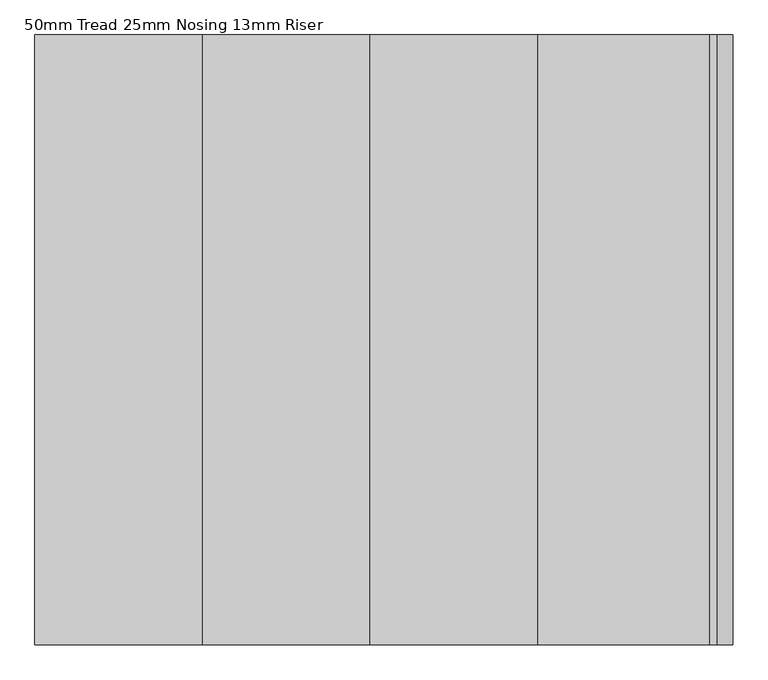
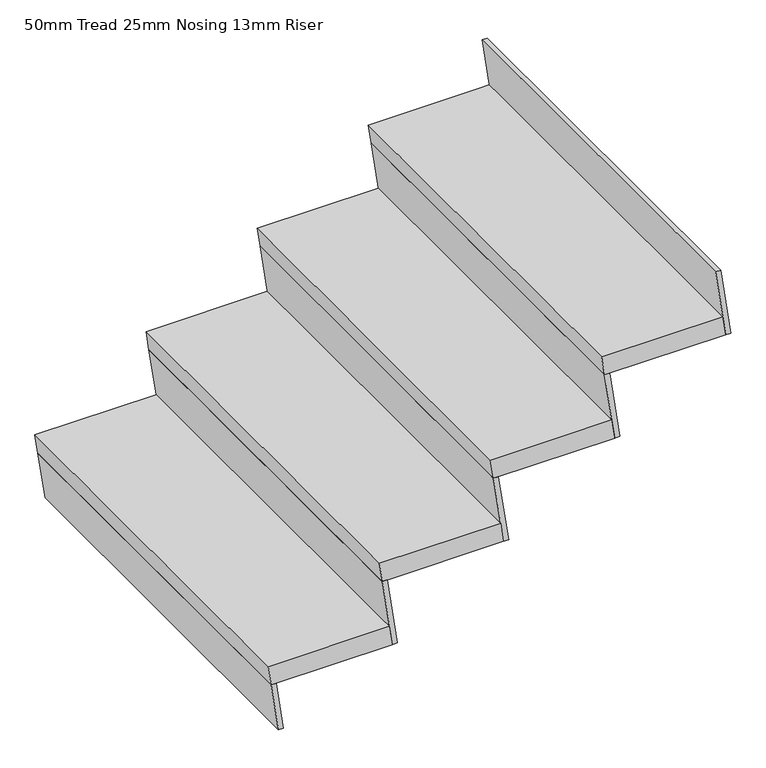
"""IFC4 building model written with IfcOpenShell, lengths in millimetres: stair flight geometry, 50mm Tread 25mm Nosing 13mm Riser."""

from ifc_helpers import new_model, si_unit, origin, place, context, project, spatial, faceted_brep, source, transform, mapped, element, save


def stair_flight_50mm_tread_25mm_nosing_13mm_riser_3ceddbfd(model_context):
    return source(origin(), model_context, "Body", "Brep", [
        faceted_brep([(-3491.9701746, -2541.1890637, 173.9130435), (-3484.7826746, -2541.1890637, 123.9130435), (-3484.7826746, -1541.1632824, 123.9130435), (-3491.9701746, -1541.1632824, 173.9130435), (-3791.9701746, -1541.1632824, 173.9130435), (-3791.9701746, -2541.1890637, 173.9130435), (-3784.7826746, -2541.1890637, 123.9130435), (-3784.7826746, -1541.1632824, 123.9130435)], [[[0, 1, 2, 3]], [[3, 4, 5, 0]], [[2, 1, 6, 7]], [[4, 3, 2, 7]], [[0, 5, 6, 1]], [[5, 4, 7, 6]]]),
        faceted_brep([(-3784.7826746, -2541.1890637, 123.9130435), (-3766.9701746, -2541.1890637, 0.0), (-3754.3416846, -2541.1890637, 0.0), (-3772.1541846, -2541.1890637, 123.9130435), (-3784.7826746, -1541.1632824, 123.9130435), (-3772.1541846, -1541.1632824, 123.9130435), (-3754.3416846, -1541.1632824, 0.0), (-3766.9701746, -1541.1632824, 0.0)], [[[0, 1, 2, 3]], [[4, 5, 6, 7]], [[1, 0, 4, 7]], [[2, 1, 7, 6]], [[3, 2, 6, 5]], [[0, 3, 5, 4]]]),
        faceted_brep([(-3509.7826746, -2541.1890637, 297.826087), (-3484.7826746, -2541.1890637, 123.9130435), (-3472.1541846, -2541.1890637, 123.9130435), (-3497.1541846, -2541.1890637, 297.826087), (-3509.7826746, -1541.1632824, 297.826087), (-3497.1541846, -1541.1632824, 297.826087), (-3472.1541846, -1541.1632824, 123.9130435), (-3484.7826746, -1541.1632824, 123.9130435)], [[[0, 1, 2, 3]], [[4, 5, 6, 7]], [[1, 0, 4, 7]], [[2, 1, 7, 6]], [[3, 2, 6, 5]], [[0, 3, 5, 4]]]),
        faceted_brep([(-3216.9701746, -1541.1632824, 347.826087), (-3516.9701746, -1541.1632824, 347.826087), (-3516.9701746, -2541.1890637, 347.826087), (-3216.9701746, -2541.1890637, 347.826087), (-3209.7826746, -1541.1632824, 297.826087), (-3209.7826746, -2541.1890637, 297.826087), (-3509.7826746, -2541.1890637, 297.826087), (-3509.7826746, -1541.1632824, 297.826087)], [[[0, 1, 2, 3]], [[4, 5, 6, 7]], [[1, 0, 4, 7]], [[3, 2, 6, 5]], [[3, 5, 4, 0]], [[2, 1, 7, 6]]]),
        faceted_brep([(-3234.7826746, -2541.1890637, 471.7391304), (-3209.7826746, -2541.1890637, 297.826087), (-3197.1541846, -2541.1890637, 297.826087), (-3222.1541846, -2541.1890637, 471.7391304), (-3234.7826746, -1541.1632824, 471.7391304), (-3222.1541846, -1541.1632824, 471.7391304), (-3197.1541846, -1541.1632824, 297.826087), (-3209.7826746, -1541.1632824, 297.826087)], [[[0, 1, 2, 3]], [[4, 5, 6, 7]], [[1, 0, 4, 7]], [[2, 1, 7, 6]], [[3, 2, 6, 5]], [[0, 3, 5, 4]]]),
        faceted_brep([(-2941.9701746, -1541.1632824, 521.7391304), (-3241.9701746, -1541.1632824, 521.7391304), (-3241.9701746, -2541.1890637, 521.7391304), (-2941.9701746, -2541.1890637, 521.7391304), (-2934.7826746, -1541.1632824, 471.7391304), (-2934.7826746, -2541.1890637, 471.7391304), (-3234.7826746, -2541.1890637, 471.7391304), (-3234.7826746, -1541.1632824, 471.7391304)], [[[0, 1, 2, 3]], [[4, 5, 6, 7]], [[1, 0, 4, 7]], [[3, 2, 6, 5]], [[3, 5, 4, 0]], [[2, 1, 7, 6]]]),
        faceted_brep([(-2684.7826746, -2541.1890637, 819.5652174), (-2659.7826746, -2541.1890637, 645.6521739), (-2647.1541846, -2541.1890637, 645.6521739), (-2672.1541846, -2541.1890637, 819.5652174), (-2684.7826746, -1541.1632824, 819.5652174), (-2672.1541846, -1541.1632824, 819.5652174), (-2647.1541846, -1541.1632824, 645.6521739), (-2659.7826746, -1541.1632824, 645.6521739)], [[[0, 1, 2, 3]], [[4, 5, 6, 7]], [[1, 0, 4, 7]], [[2, 1, 7, 6]], [[3, 2, 6, 5]], [[0, 3, 5, 4]]]),
        faceted_brep([(-2959.7826746, -2541.1890637, 645.6521739), (-2934.7826746, -2541.1890637, 471.7391304), (-2922.1541846, -2541.1890637, 471.7391304), (-2947.1541846, -2541.1890637, 645.6521739), (-2959.7826746, -1541.1632824, 645.6521739), (-2947.1541846, -1541.1632824, 645.6521739), (-2922.1541846, -1541.1632824, 471.7391304), (-2934.7826746, -1541.1632824, 471.7391304)], [[[0, 1, 2, 3]], [[4, 5, 6, 7]], [[1, 0, 4, 7]], [[2, 1, 7, 6]], [[3, 2, 6, 5]], [[0, 3, 5, 4]]]),
        faceted_brep([(-2666.9701746, -1541.1632824, 695.6521739), (-2691.9701746, -1541.1632824, 695.6521739), (-2966.9701746, -1541.1632824, 695.6521739), (-2966.9701746, -2541.1890637, 695.6521739), (-2666.9701746, -2541.1890637, 695.6521739), (-2659.7826746, -1541.1632824, 645.6521739), (-2659.7826746, -2541.1890637, 645.6521739), (-2959.7826746, -2541.1890637, 645.6521739), (-2959.7826746, -1541.1632824, 645.6521739), (-2691.9701746, -1541.1632824, 645.6521739)], [[[0, 1, 2, 3, 4]], [[5, 6, 7, 8, 9]], [[1, 0, 5, 9]], [[2, 1, 9, 8]], [[4, 3, 7, 6]], [[4, 6, 5, 0]], [[3, 2, 8, 7]]]),
    ])


if __name__ == "__main__":
    model = new_model("IFC4")
    model_context = context("Model", 3, world=origin())
    ifc_project = project(units=[si_unit("LENGTHUNIT", "METRE", prefix="MILLI")], contexts=[model_context])
    site = spatial("IfcSite", under=ifc_project)
    building = spatial("IfcBuilding", under=site)
    placement = place(None, origin())
    stair_flight_50mm_tread_25mm_nosing_13mm_riser_shape = stair_flight_50mm_tread_25mm_nosing_13mm_riser_3ceddbfd(model_context)
    element("IfcStairFlight", 1, ObjectType="50mm Tread 25mm Nosing 13mm Riser", at=placement, inside=building, context=model_context, shape_type="MappedRepresentation", body=[
        mapped(stair_flight_50mm_tread_25mm_nosing_13mm_riser_shape, transform((0.0, 0.0, 0.0), x_axis=(1.0, 0.0, 0.0), y_axis=(0.0, 1.0, 0.0), z_axis=(0.0, 0.0, 1.0))),
    ])
    save(model, "model.ifc")
